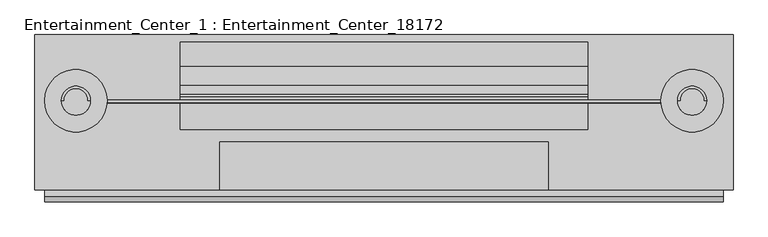
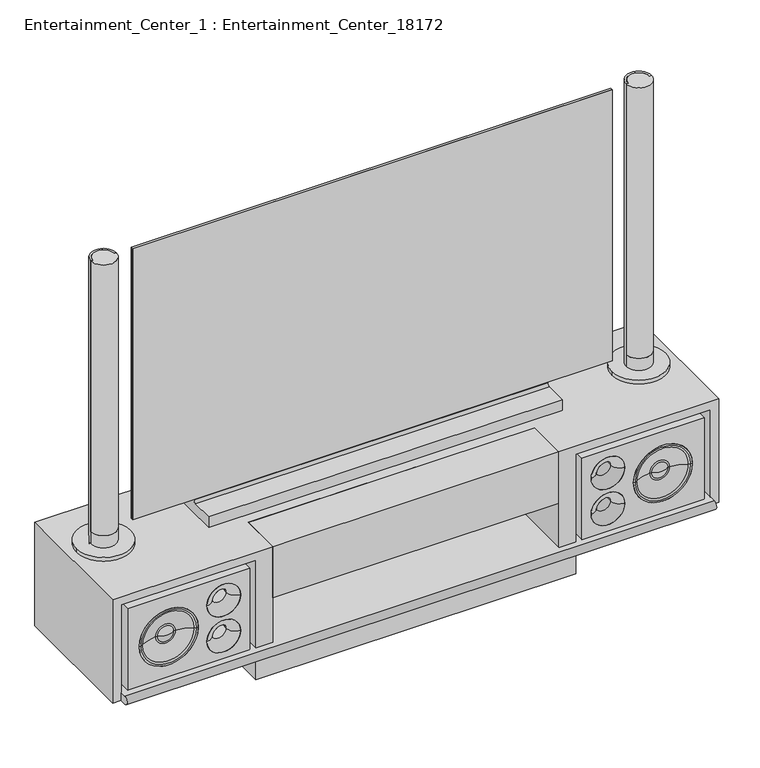
"""IFC4 building model written with IfcOpenShell, lengths in millimetres: furniture geometry, Entertainment_Center_1 : Entertainment_Center_18172."""

from ifc_helpers import new_model, si_unit, point, frame, frame_2d, origin, origin_with_axes, place, context, project, spatial, polyline, circle_curve, ellipse_curve, trimmed, segment, composite_curve, outline, extrude, faceted_brep, source, transform, mapped, element, save
from ifc_brep_helpers import plane_surface, cylinder_surface, revolved_surface, advanced_brep


def entertainment_center_1_entertainment_center_18172_277d4ec1(model_context):
    return source(origin(), model_context, "Body", "SolidModel", [
        faceted_brep([(-914.4, -406.4, 406.4), (-914.4, 0.0, 406.4), (-914.4, 0.0, 76.2), (-914.4, -406.4, 76.2), (914.4, -406.4, 406.4), (914.4, -406.4, 76.2), (914.4, 0.0, 76.2), (914.4, 0.0, 406.4), (-889.0, -406.4, 76.2), (-889.0, -406.4, 381.0), (-482.6, -406.4, 381.0), (-482.6, -406.4, 76.2), (-431.8, -406.4, 76.2), (-431.8, -406.4, 406.4), (431.8, -406.4, 406.4), (431.8, -406.4, 76.2), (482.6, -406.4, 76.2), (482.6, -406.4, 381.0), (889.0, -406.4, 381.0), (889.0, -406.4, 76.2), (889.0, -25.4, 76.2), (482.6, -25.4, 76.2), (431.8, -25.4, 76.2), (-431.8, -25.4, 76.2), (-482.6, -25.4, 76.2), (-889.0, -25.4, 76.2), (-431.8, -279.1188103, 406.4), (431.8, -279.1188103, 406.4), (-889.0, -25.4, 381.0), (-482.6, -25.4, 381.0), (889.0, -25.4, 381.0), (482.6, -25.4, 381.0), (-431.8, -25.4, 381.0), (-431.8, -279.1188103, 381.0), (431.8, -25.4, 381.0), (431.8, -279.1188103, 381.0)], [[[0, 1, 2, 3]], [[4, 5, 6, 7]], [[0, 3, 8, 9, 10, 11, 12, 13]], [[5, 4, 14, 15, 16, 17, 18, 19]], [[3, 2, 6, 5, 19, 20, 21, 16, 15, 22, 23, 12, 11, 24, 25, 8]], [[2, 1, 7, 6]], [[1, 0, 13, 26, 27, 14, 4, 7]], [[28, 9, 8, 25]], [[29, 24, 11, 10]], [[9, 28, 29, 10]], [[28, 25, 24, 29]], [[30, 20, 19, 18]], [[31, 17, 16, 21]], [[30, 18, 17, 31]], [[20, 30, 31, 21]], [[23, 32, 33, 26, 13, 12]], [[34, 22, 15, 14, 27, 35]], [[32, 34, 35, 33]], [[32, 23, 22, 34]], [[26, 33, 35, 27]]]),
        extrude(outline(composite_curve([segment(trimmed(circle_curve(frame_2d((-425.45, 88.9)), 12.7), [point((-425.45, 76.2))], [point((-425.45, 101.6))], False, "CARTESIAN"), True, "CONTINUOUS"), segment(polyline([(-425.45, 101.6), (-25.4, 101.6), (-25.4, 76.2), (-425.45, 76.2)]), True, "CONTINUOUS")], self_intersect=False)), frame((-889.0, 0.0, 0.0), z_axis=(1.0, 0.0, 0.0), x_axis=(0.0, 1.0, 0.0)), (0.0, 0.0, 1.0), 1778.0),
        extrude(outline(polyline([(-431.8, -25.4), (431.8, -25.4), (431.8, -368.0188103), (-431.8, -368.0188103), (-431.8, -25.4)])), frame((0.0, 0.0, 241.3), z_axis=(0.0, 0.0, 1.0), x_axis=(1.0, 0.0, 0.0)), (0.0, 0.0, 1.0), 10.9060017),
        extrude(outline(polyline([(-406.4, 406.4), (-279.1188103, 406.4), (-279.1188103, 400.05), (-400.05, 400.05), (-400.05, 243.0276949), (-406.4, 243.0276949), (-406.4, 406.4)])), frame((-431.8, 0.0, 0.0), z_axis=(1.0, 0.0, 0.0), x_axis=(0.0, 1.0, 0.0)), (0.0, 0.0, 1.0), 863.6),
        extrude(outline(polyline([(482.6, -25.4), (482.6, -406.4), (-482.6, -406.4), (-482.6, -25.4), (482.6, -25.4)])), origin_with_axes(), (0.0, 0.0, 1.0), 76.2),
        extrude(outline(polyline([(-723.4590197, -171.5160674), (723.4590197, -171.5160674), (723.4590197, -177.8660674), (-723.4590197, -177.8660674), (-723.4590197, -171.5160674)])), frame((0.0, 0.0, 457.2), z_axis=(0.0, 0.0, 1.0), x_axis=(1.0, 0.0, 0.0)), (0.0, 0.0, 1.0), 863.6),
        extrude(outline(composite_curve([segment(polyline([(-247.7160674, 441.1123847), (-179.0392237, 441.1123847)]), True, "CONTINUOUS"), segment(trimmed(circle_curve(frame_2d((-179.0392237, 448.6355411)), 7.5231564), [point((-179.0392237, 441.1123847))], [point((-171.5160674, 448.6355411))], True, "CARTESIAN"), True, "CONTINUOUS"), segment(polyline([(-171.5160674, 448.6355411), (-171.5160674, 658.3840106), (-161.5837628, 658.3840106), (-155.1782559, 640.7850249)]), True, "CONTINUOUS"), segment(trimmed(circle_curve(frame_2d((-495.3, 516.9908341)), 361.95), [point((-155.1782559, 640.7850249))], [point((-133.35, 516.9908341))], False, "CARTESIAN"), True, "CONTINUOUS"), segment(polyline([(-133.35, 516.9908341), (-133.35, 491.9123847)]), True, "CONTINUOUS"), segment(trimmed(circle_curve(frame_2d((-82.55, 491.9123847)), 50.8), [point((-133.35, 491.9123847))], [point((-82.55, 441.1123847))], True, "CARTESIAN"), True, "CONTINUOUS"), segment(polyline([(-82.55, 441.1123847), (-19.05, 441.1123847), (-19.05, 406.4), (-247.7160674, 406.4), (-247.7160674, 441.1123847)]), True, "CONTINUOUS")], self_intersect=False)), frame((-533.4, 0.0, 0.0), z_axis=(1.0, 0.0, 0.0), x_axis=(0.0, 1.0, 0.0)), (0.0, 0.0, 1.0), 1066.8),
        extrude(outline(polyline([(723.4590197, -179.4295839), (-723.4590197, -179.4295839), (-723.4590197, -175.7159791), (723.4590197, -175.7159791), (723.4590197, -179.4295839)])), frame((0.0, 0.0, 457.2), z_axis=(0.0, 0.0, 1.0), x_axis=(1.0, 0.0, 0.0)), (0.0, 0.0, 1.0), 863.6),
        advanced_brep(
        [(-845.3548485, -172.8664931, 406.4), (-769.1548485, -172.8664931, 406.4), (-769.1548485, -172.8664931, 1320.8), (-845.3548485, -172.8664931, 1320.8), (-839.0048485, -172.8664931, 1320.8), (-775.5048485, -172.8664931, 1320.8), (-845.3548485, -172.8664931, 457.2), (-769.1548485, -172.8664931, 457.2), (-839.0048485, -172.8664931, 457.2), (-775.5048485, -172.8664931, 457.2)],
        [
            (0, 1, circle_curve(frame((-807.2548485, -172.8664931, 406.4), z_axis=(0.0, 0.0, -1.0), x_axis=(1.0, 0.0, 0.0)), 38.1)),
            (1, 0, circle_curve(frame((-807.2548485, -172.8664931, 406.4), z_axis=(0.0, 0.0, -1.0), x_axis=(1.0, 0.0, 0.0)), 38.1)),
            (2, 3, circle_curve(frame((-807.2548485, -172.8664931, 1320.8), z_axis=(0.0, 0.0, 1.0), x_axis=(1.0, 0.0, 0.0)), 38.1)),
            (3, 4),
            (4, 5, circle_curve(frame((-807.2548485, -172.8664931, 1320.8), z_axis=(0.0, 0.0, -1.0), x_axis=(1.0, 0.0, 0.0)), 31.75)),
            (5, 2),
            (0, 6),
            (6, 3),
            (2, 7),
            (7, 1),
            (7, 6, circle_curve(frame((-807.2548485, -172.8664931, 457.2), z_axis=(0.0, 0.0, -1.0), x_axis=(1.0, 0.0, 0.0)), 38.1)),
            (8, 6),
            (7, 9),
            (9, 8, circle_curve(frame((-807.2548485, -172.8664931, 457.2), z_axis=(0.0, 0.0, 1.0), x_axis=(1.0, 0.0, 0.0)), 31.75)),
            (8, 4),
            (5, 9),
        ],
        [
            plane_surface(frame((-812.8, 0.0, 406.4), z_axis=(0.0, 0.0, -1.0), x_axis=(0.0, -1.0, 0.0))),
            plane_surface(frame((-812.8, 0.0, 1320.8), z_axis=(0.0, 0.0, 1.0), x_axis=(0.0, -1.0, 0.0))),
            cylinder_surface(frame((-807.2548485, -172.8664931, 406.4), z_axis=(0.0, 0.0, -1.0), x_axis=(1.0, 0.0, 0.0)), 38.1),
            plane_surface(frame((-807.2548485, 0.0, 457.2), z_axis=(0.0, 0.0, 1.0), x_axis=(0.0, -1.0, 0.0))),
            plane_surface(frame((-839.0048485, -172.8664931, 1320.8), z_axis=(0.0, -1.0, 0.0), x_axis=(0.0, 0.0, -1.0))),
            plane_surface(frame((-769.1548485, -172.8664931, 1320.8), z_axis=(0.0, -1.0, 0.0), x_axis=(0.0, 0.0, -1.0))),
            revolved_surface(polyline([(-775.5048485, -172.8664931, 1320.8), (-775.5048485, -172.8664931, 457.20000000000005)]), (-807.2548485, -172.8664931, 1320.8), (0.0, 0.0, 1.0)),
        ],
        [
            (0, [[1, 2]]),
            (1, [[3, 4, 5, 6]]),
            (2, [[-1, 7, 8, -3, 9, 10]]),
            (2, [[-2, -10, 11, -7]]),
            (3, [[12, -11, 13, 14]]),
            (4, [[-12, 15, -4, -8]]),
            (5, [[-13, -9, -6, 16]]),
            (6, [[-14, -16, -5, -15]]),
        ],
    ),
        extrude(outline(composite_curve([segment(trimmed(circle_curve(frame_2d((-807.2548485, -172.8664931)), 81.7451515), [point((-889.0, -172.8664931))], [point((-725.509697, -172.8664931))], False, "CARTESIAN"), True, "CONTINUOUS"), segment(trimmed(circle_curve(frame_2d((-807.2548485, -172.8664931)), 81.7451515), [point((-725.509697, -172.8664931))], [point((-889.0, -172.8664931))], False, "CARTESIAN"), True, "CONTINUOUS")], self_intersect=False)), frame((0.0, 0.0, 406.4), z_axis=(0.0, 0.0, 1.0), x_axis=(1.0, 0.0, 0.0)), (0.0, 0.0, 1.0), 12.7),
        extrude(outline(composite_curve([segment(trimmed(circle_curve(frame_2d((807.2548485, -172.8664931)), 81.7451515), [point((889.0, -172.8664931))], [point((725.509697, -172.8664931))], False, "CARTESIAN"), True, "CONTINUOUS"), segment(trimmed(circle_curve(frame_2d((807.2548485, -172.8664931)), 81.7451515), [point((725.509697, -172.8664931))], [point((889.0, -172.8664931))], False, "CARTESIAN"), True, "CONTINUOUS")], self_intersect=False)), frame((0.0, 0.0, 406.4), z_axis=(0.0, 0.0, 1.0), x_axis=(1.0, 0.0, 0.0)), (0.0, 0.0, 1.0), 12.7),
        extrude(outline(composite_curve([segment(trimmed(circle_curve(frame_2d((-807.2548485, -172.8664931)), 38.1), [point((-769.1548485, -172.8664931))], [point((-845.3548485, -172.8664931))], False, "CARTESIAN"), True, "CONTINUOUS"), segment(polyline([(-845.3548485, -172.8664931), (-839.0048485, -172.8664931)]), True, "CONTINUOUS"), segment(trimmed(circle_curve(frame_2d((-807.2548485, -172.8664931)), 31.75), [point((-839.0048485, -172.8664931))], [point((-775.5048485, -172.8664931))], False, "CARTESIAN"), True, "CONTINUOUS"), segment(polyline([(-775.5048485, -172.8664931), (-769.1548485, -172.8664931)]), True, "CONTINUOUS")], self_intersect=False)), frame((0.0, 0.0, 457.2), z_axis=(0.0, 0.0, 1.0), x_axis=(1.0, 0.0, 0.0)), (0.0, 0.0, 1.0), 863.6),
        advanced_brep(
        [(845.3548485, -172.8664931, 406.4), (769.1548485, -172.8664931, 406.4), (845.3548485, -172.8664931, 1320.8), (769.1548485, -172.8664931, 1320.8), (775.5048485, -172.8664931, 1320.8), (839.0048485, -172.8664931, 1320.8), (769.1548485, -172.8664931, 457.2), (845.3548485, -172.8664931, 457.2), (839.0048485, -172.8664931, 457.2), (775.5048485, -172.8664931, 457.2)],
        [
            (0, 1, circle_curve(frame((807.2548485, -172.8664931, 406.4), z_axis=(0.0, 0.0, -1.0), x_axis=(-1.0, 0.0, 0.0)), 38.1)),
            (1, 0, circle_curve(frame((807.2548485, -172.8664931, 406.4), z_axis=(0.0, 0.0, -1.0), x_axis=(-1.0, 0.0, 0.0)), 38.1)),
            (2, 3, circle_curve(frame((807.2548485, -172.8664931, 1320.8), z_axis=(0.0, 0.0, 1.0), x_axis=(-1.0, 0.0, 0.0)), 38.1)),
            (3, 4),
            (4, 5, circle_curve(frame((807.2548485, -172.8664931, 1320.8), z_axis=(0.0, 0.0, -1.0), x_axis=(-1.0, 0.0, 0.0)), 31.75)),
            (5, 2),
            (1, 6),
            (6, 3),
            (2, 7),
            (7, 0),
            (7, 6, circle_curve(frame((807.2548485, -172.8664931, 457.2), z_axis=(0.0, 0.0, -1.0), x_axis=(-1.0, 0.0, 0.0)), 38.1)),
            (8, 9, circle_curve(frame((807.2548485, -172.8664931, 457.2), z_axis=(0.0, 0.0, 1.0), x_axis=(-1.0, 0.0, 0.0)), 31.75)),
            (9, 6),
            (7, 8),
            (5, 8),
            (9, 4),
        ],
        [
            plane_surface(frame((812.8, 0.0, 406.4), z_axis=(0.0, 0.0, -1.0), x_axis=(0.0, 1.0, 0.0))),
            plane_surface(frame((812.8, 0.0, 1320.8), z_axis=(0.0, 0.0, 1.0), x_axis=(0.0, 1.0, 0.0))),
            cylinder_surface(frame((807.2548485, -172.8664931, 406.4), z_axis=(0.0, 0.0, -1.0), x_axis=(-1.0, 0.0, 0.0)), 38.1),
            plane_surface(frame((807.2548485, 0.0, 457.2), z_axis=(0.0, 0.0, 1.0), x_axis=(0.0, 1.0, 0.0))),
            plane_surface(frame((845.3548485, -172.8664931, 1320.8), z_axis=(0.0, -1.0, 0.0), x_axis=(0.0, 0.0, -1.0))),
            plane_surface(frame((775.5048485, -172.8664931, 1320.8), z_axis=(0.0, -1.0, 0.0), x_axis=(0.0, 0.0, -1.0))),
            revolved_surface(polyline([(775.5048485, -172.8664931, 1320.8), (775.5048485, -172.8664931, 457.20000000000005)]), (807.2548485, -172.8664931, 1320.8), (0.0, 0.0, 1.0)),
        ],
        [
            (0, [[1, 2]]),
            (1, [[3, 4, 5, 6]]),
            (2, [[-2, 7, 8, -3, 9, 10]]),
            (2, [[-1, -10, 11, -7]]),
            (3, [[12, 13, -11, 14]]),
            (4, [[-14, -9, -6, 15]]),
            (5, [[-13, 16, -4, -8]]),
            (6, [[-12, -15, -5, -16]]),
        ],
    ),
        extrude(outline(composite_curve([segment(trimmed(circle_curve(frame_2d((807.2548485, -172.8664931)), 38.1), [point((845.3548485, -172.8664931))], [point((769.1548485, -172.8664931))], False, "CARTESIAN"), True, "CONTINUOUS"), segment(polyline([(769.1548485, -172.8664931), (775.5048485, -172.8664931)]), True, "CONTINUOUS"), segment(trimmed(circle_curve(frame_2d((807.2548485, -172.8664931)), 31.75), [point((775.5048485, -172.8664931))], [point((839.0048485, -172.8664931))], False, "CARTESIAN"), True, "CONTINUOUS"), segment(polyline([(839.0048485, -172.8664931), (845.3548485, -172.8664931)]), True, "CONTINUOUS")], self_intersect=False)), frame((0.0, 0.0, 457.2), z_axis=(0.0, 0.0, 1.0), x_axis=(1.0, 0.0, 0.0)), (0.0, 0.0, 1.0), 863.6),
        extrude(outline(polyline([(-191.3302869, -321.3336205), (-191.3302869, -73.6836205), (189.6697131, -73.6836205), (189.6697131, -321.3336205), (-191.3302869, -321.3336205)])), frame((0.0, 0.0, 264.3017952), z_axis=(0.0, 0.0, 1.0), x_axis=(1.0, 0.0, 0.0)), (0.0, 0.0, 1.0), 57.15),
        extrude(outline(polyline([(-101.6, -327.3863852), (-101.6, -276.5863852), (101.6, -276.5863852), (101.6, -327.3863852), (-101.6, -327.3863852)])), frame((0.0, 0.0, 290.7540192), z_axis=(0.0, 0.0, 1.0), x_axis=(1.0, 0.0, 0.0)), (0.0, 0.0, 1.0), 19.05),
        extrude(outline(polyline([(-501.298763, -342.9), (-869.598763, -342.9), (-869.598763, -76.2), (-501.298763, -76.2), (-501.298763, -342.9)])), frame((0.0, 0.0, 101.6), z_axis=(0.0, 0.0, 1.0), x_axis=(1.0, 0.0, 0.0)), (0.0, 0.0, 1.0), 259.8201277),
        advanced_brep(
        [(-656.4895317, -406.4, 228.6), (-834.2895317, -406.4, 228.6), (-834.2895317, -342.9, 228.6), (-656.4895317, -342.9, 228.6), (-661.4072329, -406.4, 228.6), (-829.3718304, -406.4, 228.6), (-666.9861301, -403.5094482, 228.6), (-823.7929332, -403.5094482, 228.6), (-715.3754427, -388.7524859, 228.6), (-775.4036207, -388.7524859, 228.6), (-745.3895317, -398.3592917, 228.6), (-770.1255754, -389.6831477, 228.6), (-720.653488, -389.6831477, 228.6), (-745.3895317, -342.9, 228.6)],
        [
            (0, 1, circle_curve(frame((-745.3895317, -406.4, 228.6), z_axis=(0.0, 1.0, 0.0), x_axis=(-1.0, 0.0, 0.0)), 88.9)),
            (1, 2),
            (2, 3, circle_curve(frame((-745.3895317, -342.9, 228.6), z_axis=(0.0, -1.0, 0.0), x_axis=(-1.0, 0.0, 0.0)), 88.9)),
            (3, 0),
            (1, 0, circle_curve(frame((-745.3895317, -406.4, 228.6), z_axis=(0.0, 1.0, 0.0), x_axis=(-1.0, 0.0, 0.0)), 88.9)),
            (3, 2, circle_curve(frame((-745.3895317, -342.9, 228.6), z_axis=(0.0, -1.0, 0.0), x_axis=(-1.0, 0.0, 0.0)), 88.9)),
            (4, 5, circle_curve(frame((-745.3895317, -406.4, 228.6), z_axis=(0.0, 1.0, 0.0), x_axis=(-1.0, 0.0, 0.0)), 83.9822987)),
            (5, 1),
            (0, 4),
            (5, 4, circle_curve(frame((-745.3895317, -406.4, 228.6), z_axis=(0.0, 1.0, 0.0), x_axis=(-1.0, 0.0, 0.0)), 83.9822987)),
            (6, 7, circle_curve(frame((-745.3895317, -403.5094482, 228.6), z_axis=(0.0, 1.0, 0.0), x_axis=(-1.0, 0.0, 0.0)), 78.4034016)),
            (7, 5, circle_curve(frame((-827.3631505, -403.4478049, 228.6), z_axis=(0.0, 0.0, -1.0), x_axis=(1.0, 0.0, 0.0)), 3.5707494)),
            (4, 6, circle_curve(frame((-663.4159129, -403.4478049, 228.6), z_axis=(0.0, 0.0, -1.0), x_axis=(-1.0, 0.0, 0.0)), 3.5707494)),
            (7, 6, circle_curve(frame((-745.3895317, -403.5094482, 228.6), z_axis=(0.0, 1.0, 0.0), x_axis=(-1.0, 0.0, 0.0)), 78.4034016)),
            (8, 9, circle_curve(frame((-745.3895317, -388.7524859, 228.6), z_axis=(0.0, 1.0, 0.0), x_axis=(-1.0, 0.0, 0.0)), 30.014089)),
            (9, 7, circle_curve(frame((-754.4517947, -544.1700552, 228.6), z_axis=(0.0, 0.0, 1.0), x_axis=(1.0, 0.0, 0.0)), 156.8234672)),
            (6, 8, circle_curve(frame((-736.3272687, -544.1700552, 228.6), z_axis=(0.0, 0.0, 1.0), x_axis=(-1.0, 0.0, 0.0)), 156.8234672)),
            (9, 8, circle_curve(frame((-745.3895317, -388.7524859, 228.6), z_axis=(0.0, 1.0, 0.0), x_axis=(-1.0, 0.0, 0.0)), 30.014089)),
            (10, 11, circle_curve(frame((-745.3895317, -358.7594802, 228.6), z_axis=(0.0, 0.0, -1.0), x_axis=(1.0, 0.0, 0.0)), 39.5998114)),
            (11, 12, circle_curve(frame((-745.3895317, -389.6831477, 228.6), z_axis=(0.0, -1.0, 0.0), x_axis=(-1.0, 0.0, 0.0)), 24.7360437)),
            (12, 10, circle_curve(frame((-745.3895317, -358.7594802, 228.6), z_axis=(0.0, 0.0, -1.0), x_axis=(-1.0, 0.0, 0.0)), 39.5998114)),
            (12, 11, circle_curve(frame((-745.3895317, -389.6831477, 228.6), z_axis=(0.0, -1.0, 0.0), x_axis=(-1.0, 0.0, 0.0)), 24.7360437)),
            (2, 13),
            (13, 3),
            (11, 9, circle_curve(frame((-772.5432213, -387.9623269, 228.6), z_axis=(0.0, 0.0, -1.0), x_axis=(1.0, 0.0, 0.0)), 2.9675303)),
            (8, 12, circle_curve(frame((-718.2358421, -387.9623269, 228.6), z_axis=(0.0, 0.0, -1.0), x_axis=(-1.0, 0.0, 0.0)), 2.9675303)),
        ],
        [
            cylinder_surface(frame((-745.3895317, -391.7344921, 228.6), z_axis=(0.0, -1.0, 0.0), x_axis=(-1.0, 0.0, 0.0)), 88.9),
            plane_surface(frame((-745.3895317, -406.4, 228.6), z_axis=(0.0, -1.0, 0.0), x_axis=(-1.0, 0.0, 0.0))),
            revolved_surface(trimmed(ellipse_curve(frame((-827.3631505, -403.4478049, 228.6), z_axis=(0.0, 0.0, 1.0), x_axis=(1.0, 0.0, 0.0)), 3.5707494, 3.5707494), [point((-829.3718304, -406.4, 228.6))], [point((-823.7929332, -403.5094482, 228.6))], True, "CARTESIAN"), (-745.3895317, -391.7344921, 228.6), (0.0, -1.0, 0.0)),
            revolved_surface(trimmed(ellipse_curve(frame((-754.4517947, -544.1700552, 228.6), z_axis=(0.0, 0.0, -1.0), x_axis=(1.0, 0.0, 0.0)), 156.8234672, 156.8234672), [point((-823.7929332, -403.5094482, 228.6))], [point((-775.4036207, -388.7524859, 228.6))], True, "CARTESIAN"), (-745.3895317, -391.7344921, 228.6), (0.0, -1.0, 0.0)),
            revolved_surface(trimmed(ellipse_curve(frame((-745.3895317, -358.7594802, 228.6), z_axis=(0.0, 0.0, 1.0), x_axis=(1.0, 0.0, 0.0)), 39.5998114, 39.5998114), [point((-770.1255754, -389.6831477, 228.6))], [point((-745.3895317, -398.3592917, 228.6))], True, "CARTESIAN"), (-745.3895317, -391.7344921, 228.6), (0.0, -1.0, 0.0)),
            plane_surface(frame((-745.3895317, -342.9, 228.6), z_axis=(0.0, 1.0, 0.0), x_axis=(-1.0, 0.0, 0.0))),
            revolved_surface(trimmed(ellipse_curve(frame((-772.5432213, -387.9623269, 228.6), z_axis=(0.0, 0.0, 1.0), x_axis=(1.0, 0.0, 0.0)), 2.9675303, 2.9675303), [point((-775.4036207, -388.7524859, 228.6))], [point((-770.1255754, -389.6831477, 228.6))], True, "CARTESIAN"), (-745.3895317, -391.7344921, 228.6), (0.0, -1.0, 0.0)),
        ],
        [
            (0, [[1, 2, 3, 4]]),
            (0, [[5, -4, 6, -2]]),
            (1, [[7, 8, -1, 9]]),
            (1, [[10, -9, -5, -8]]),
            (2, [[11, 12, -7, 13]]),
            (2, [[14, -13, -10, -12]]),
            (3, [[15, 16, -11, 17]]),
            (3, [[18, -17, -14, -16]]),
            (4, [[19, 20, 21]]),
            (4, [[-21, 22, -19]]),
            (5, [[-3, 23, 24]]),
            (5, [[-6, -24, -23]]),
            (6, [[-20, 25, -15, 26]]),
            (6, [[-22, -26, -18, -25]]),
        ],
    ),
        extrude(outline(polyline([(361.4201277, -501.298763), (361.4201277, -869.598763), (101.6, -869.598763), (101.6, -501.298763), (361.4201277, -501.298763)]), holes=[composite_curve([segment(trimmed(circle_curve(frame_2d((228.6, -745.3895317)), 88.9), [point((228.6, -834.2895317))], [point((228.6, -656.4895317))], True, "CARTESIAN"), True, "CONTINUOUS"), segment(trimmed(circle_curve(frame_2d((228.6, -745.3895317)), 88.9), [point((228.6, -656.4895317))], [point((228.6, -834.2895317))], True, "CARTESIAN"), True, "CONTINUOUS")], self_intersect=False), composite_curve([segment(trimmed(circle_curve(frame_2d((173.1686264, -579.5939749)), 50.8), [point((173.1686264, -630.3939749))], [point((173.1686264, -528.7939749))], True, "CARTESIAN"), True, "CONTINUOUS"), segment(trimmed(circle_curve(frame_2d((173.1686264, -579.5939749)), 50.8), [point((173.1686264, -528.7939749))], [point((173.1686264, -630.3939749))], True, "CARTESIAN"), True, "CONTINUOUS")], self_intersect=False), composite_curve([segment(trimmed(circle_curve(frame_2d((287.4686264, -579.5939749)), 50.8), [point((287.4686264, -630.3939749))], [point((287.4686264, -528.7939749))], True, "CARTESIAN"), True, "CONTINUOUS"), segment(trimmed(circle_curve(frame_2d((287.4686264, -579.5939749)), 50.8), [point((287.4686264, -528.7939749))], [point((287.4686264, -630.3939749))], True, "CARTESIAN"), True, "CONTINUOUS")], self_intersect=False)]), frame((0.0, -406.4, 0.0), z_axis=(0.0, 1.0, 0.0), x_axis=(0.0, 0.0, 1.0)), (0.0, 0.0, 1.0), 63.5),
        advanced_brep(
        [(-554.8020523, -342.9, 173.1686264), (-604.3858975, -342.9, 173.1686264), (-602.8610938, -377.9369622, 173.1686264), (-556.3268561, -377.9369622, 173.1686264), (-528.7939749, -342.9, 173.1686264), (-630.3939749, -342.9, 173.1686264), (-528.7939749, -406.4, 173.1686264), (-630.3939749, -406.4, 173.1686264)],
        [
            (0, 1, circle_curve(frame((-579.5939749, -342.9, 173.1686264), z_axis=(0.0, 1.0, 0.0), x_axis=(-1.0, 0.0, 0.0)), 24.7919226)),
            (1, 2),
            (2, 3, circle_curve(frame((-579.5939749, -377.9369622, 173.1686264), z_axis=(0.0, -1.0, 0.0), x_axis=(-1.0, 0.0, 0.0)), 23.2671189)),
            (3, 0),
            (1, 0, circle_curve(frame((-579.5939749, -342.9, 173.1686264), z_axis=(0.0, 1.0, 0.0), x_axis=(-1.0, 0.0, 0.0)), 24.7919226)),
            (3, 2, circle_curve(frame((-579.5939749, -377.9369622, 173.1686264), z_axis=(0.0, -1.0, 0.0), x_axis=(-1.0, 0.0, 0.0)), 23.2671189)),
            (4, 5, circle_curve(frame((-579.5939749, -342.9, 173.1686264), z_axis=(0.0, 1.0, 0.0), x_axis=(-1.0, 0.0, 0.0)), 50.8)),
            (5, 1),
            (0, 4),
            (5, 4, circle_curve(frame((-579.5939749, -342.9, 173.1686264), z_axis=(0.0, 1.0, 0.0), x_axis=(-1.0, 0.0, 0.0)), 50.8)),
            (6, 7, circle_curve(frame((-579.5939749, -406.4, 173.1686264), z_axis=(0.0, 1.0, 0.0), x_axis=(-1.0, 0.0, 0.0)), 50.8)),
            (7, 5),
            (4, 6),
            (7, 6, circle_curve(frame((-579.5939749, -406.4, 173.1686264), z_axis=(0.0, 1.0, 0.0), x_axis=(-1.0, 0.0, 0.0)), 50.8)),
            (2, 7, circle_curve(frame((-630.1137437, -379.1229937, 173.1686264), z_axis=(0.0, 0.0, -1.0), x_axis=(1.0, 0.0, 0.0)), 27.2784457)),
            (6, 3, circle_curve(frame((-529.0742061, -379.1229937, 173.1686264), z_axis=(0.0, 0.0, -1.0), x_axis=(-1.0, 0.0, 0.0)), 27.2784457)),
        ],
        [
            revolved_surface(polyline([(-602.8610938, -377.9369622, 173.1686264), (-604.3858975, -342.9, 173.1686264)]), (-579.5939749, -374.65, 173.1686264), (0.0, -1.0, 0.0)),
            plane_surface(frame((-579.5939749, -342.9, 173.1686264), z_axis=(0.0, 1.0, 0.0), x_axis=(-1.0, 0.0, 0.0))),
            cylinder_surface(frame((-579.5939749, -374.65, 173.1686264), z_axis=(0.0, -1.0, 0.0), x_axis=(-1.0, 0.0, 0.0)), 50.8),
            revolved_surface(trimmed(ellipse_curve(frame((-630.1137437, -379.1229937, 173.1686264), z_axis=(0.0, 0.0, 1.0), x_axis=(1.0, 0.0, 0.0)), 27.2784457, 27.2784457), [point((-630.3939749, -406.4, 173.1686264))], [point((-602.8610938, -377.9369622, 173.1686264))], True, "CARTESIAN"), (-579.5939749, -374.65, 173.1686264), (0.0, -1.0, 0.0)),
        ],
        [
            (0, [[1, 2, 3, 4]]),
            (0, [[5, -4, 6, -2]]),
            (1, [[7, 8, -1, 9]]),
            (1, [[10, -9, -5, -8]]),
            (2, [[11, 12, -7, 13]]),
            (2, [[14, -13, -10, -12]]),
            (3, [[-3, 15, -11, 16]]),
            (3, [[-6, -16, -14, -15]]),
        ],
    ),
        advanced_brep(
        [(-554.8020523, -342.9, 287.4686264), (-604.3858975, -342.9, 287.4686264), (-602.8610938, -377.9369622, 287.4686264), (-556.3268561, -377.9369622, 287.4686264), (-528.7939749, -342.9, 287.4686264), (-630.3939749, -342.9, 287.4686264), (-528.7939749, -406.4, 287.4686264), (-630.3939749, -406.4, 287.4686264)],
        [
            (0, 1, circle_curve(frame((-579.5939749, -342.9, 287.4686264), z_axis=(0.0, 1.0, 0.0), x_axis=(-1.0, 0.0, 0.0)), 24.7919226)),
            (1, 2),
            (2, 3, circle_curve(frame((-579.5939749, -377.9369622, 287.4686264), z_axis=(0.0, -1.0, 0.0), x_axis=(-1.0, 0.0, 0.0)), 23.2671189)),
            (3, 0),
            (1, 0, circle_curve(frame((-579.5939749, -342.9, 287.4686264), z_axis=(0.0, 1.0, 0.0), x_axis=(-1.0, 0.0, 0.0)), 24.7919226)),
            (3, 2, circle_curve(frame((-579.5939749, -377.9369622, 287.4686264), z_axis=(0.0, -1.0, 0.0), x_axis=(-1.0, 0.0, 0.0)), 23.2671189)),
            (4, 5, circle_curve(frame((-579.5939749, -342.9, 287.4686264), z_axis=(0.0, 1.0, 0.0), x_axis=(-1.0, 0.0, 0.0)), 50.8)),
            (5, 1),
            (0, 4),
            (5, 4, circle_curve(frame((-579.5939749, -342.9, 287.4686264), z_axis=(0.0, 1.0, 0.0), x_axis=(-1.0, 0.0, 0.0)), 50.8)),
            (6, 7, circle_curve(frame((-579.5939749, -406.4, 287.4686264), z_axis=(0.0, 1.0, 0.0), x_axis=(-1.0, 0.0, 0.0)), 50.8)),
            (7, 5),
            (4, 6),
            (7, 6, circle_curve(frame((-579.5939749, -406.4, 287.4686264), z_axis=(0.0, 1.0, 0.0), x_axis=(-1.0, 0.0, 0.0)), 50.8)),
            (2, 7, circle_curve(frame((-630.1137437, -379.1229937, 287.4686264), z_axis=(0.0, 0.0, -1.0), x_axis=(1.0, 0.0, 0.0)), 27.2784457)),
            (6, 3, circle_curve(frame((-529.0742061, -379.1229937, 287.4686264), z_axis=(0.0, 0.0, -1.0), x_axis=(-1.0, 0.0, 0.0)), 27.2784457)),
        ],
        [
            revolved_surface(polyline([(-602.8610938, -377.9369622, 287.4686264), (-604.3858975, -342.9, 287.4686264)]), (-579.5939749, -374.65, 287.4686264), (0.0, -1.0, 0.0)),
            plane_surface(frame((-579.5939749, -342.9, 287.4686264), z_axis=(0.0, 1.0, 0.0), x_axis=(-1.0, 0.0, 0.0))),
            cylinder_surface(frame((-579.5939749, -374.65, 287.4686264), z_axis=(0.0, -1.0, 0.0), x_axis=(-1.0, 0.0, 0.0)), 50.8),
            revolved_surface(trimmed(ellipse_curve(frame((-630.1137437, -379.1229937, 287.4686264), z_axis=(0.0, 0.0, 1.0), x_axis=(1.0, 0.0, 0.0)), 27.2784457, 27.2784457), [point((-630.3939749, -406.4, 287.4686264))], [point((-602.8610938, -377.9369622, 287.4686264))], True, "CARTESIAN"), (-579.5939749, -374.65, 287.4686264), (0.0, -1.0, 0.0)),
        ],
        [
            (0, [[1, 2, 3, 4]]),
            (0, [[5, -4, 6, -2]]),
            (1, [[7, 8, -1, 9]]),
            (1, [[10, -9, -5, -8]]),
            (2, [[11, 12, -7, 13]]),
            (2, [[14, -13, -10, -12]]),
            (3, [[-3, 15, -11, 16]]),
            (3, [[-6, -16, -14, -15]]),
        ],
    ),
        extrude(outline(polyline([(869.598763, -342.9), (501.298763, -342.9), (501.298763, -76.2), (869.598763, -76.2), (869.598763, -342.9)])), frame((0.0, 0.0, 101.6), z_axis=(0.0, 0.0, 1.0), x_axis=(1.0, 0.0, 0.0)), (0.0, 0.0, 1.0), 259.8201277),
        advanced_brep(
        [(656.4895317, -342.9, 228.6), (834.2895317, -342.9, 228.6), (834.2895317, -406.4, 228.6), (656.4895317, -406.4, 228.6), (829.3718304, -406.4, 228.6), (661.4072329, -406.4, 228.6), (823.7929332, -403.5094482, 228.6), (666.9861301, -403.5094482, 228.6), (775.4036207, -388.7524859, 228.6), (715.3754427, -388.7524859, 228.6), (720.653488, -389.6831477, 228.6), (770.1255754, -389.6831477, 228.6), (745.3895317, -398.3592917, 228.6), (745.3895317, -342.9, 228.6)],
        [
            (0, 1, circle_curve(frame((745.3895317, -342.9, 228.6), z_axis=(0.0, -1.0, 0.0), x_axis=(1.0, 0.0, 0.0)), 88.9)),
            (1, 2),
            (2, 3, circle_curve(frame((745.3895317, -406.4, 228.6), z_axis=(0.0, 1.0, 0.0), x_axis=(1.0, 0.0, 0.0)), 88.9)),
            (3, 0),
            (1, 0, circle_curve(frame((745.3895317, -342.9, 228.6), z_axis=(0.0, -1.0, 0.0), x_axis=(1.0, 0.0, 0.0)), 88.9)),
            (3, 2, circle_curve(frame((745.3895317, -406.4, 228.6), z_axis=(0.0, 1.0, 0.0), x_axis=(1.0, 0.0, 0.0)), 88.9)),
            (2, 4),
            (4, 5, circle_curve(frame((745.3895317, -406.4, 228.6), z_axis=(0.0, 1.0, 0.0), x_axis=(1.0, 0.0, 0.0)), 83.9822987)),
            (5, 3),
            (5, 4, circle_curve(frame((745.3895317, -406.4, 228.6), z_axis=(0.0, 1.0, 0.0), x_axis=(1.0, 0.0, 0.0)), 83.9822987)),
            (4, 6, circle_curve(frame((827.3631505, -403.4478049, 228.6), z_axis=(0.0, 0.0, -1.0), x_axis=(-1.0, 0.0, 0.0)), 3.5707494)),
            (6, 7, circle_curve(frame((745.3895317, -403.5094482, 228.6), z_axis=(0.0, 1.0, 0.0), x_axis=(1.0, 0.0, 0.0)), 78.4034016)),
            (7, 5, circle_curve(frame((663.4159129, -403.4478049, 228.6), z_axis=(0.0, 0.0, -1.0), x_axis=(1.0, 0.0, 0.0)), 3.5707494)),
            (7, 6, circle_curve(frame((745.3895317, -403.5094482, 228.6), z_axis=(0.0, 1.0, 0.0), x_axis=(1.0, 0.0, 0.0)), 78.4034016)),
            (6, 8, circle_curve(frame((754.4517947, -544.1700552, 228.6), z_axis=(0.0, 0.0, 1.0), x_axis=(-1.0, 0.0, 0.0)), 156.8234672)),
            (8, 9, circle_curve(frame((745.3895317, -388.7524859, 228.6), z_axis=(0.0, 1.0, 0.0), x_axis=(1.0, 0.0, 0.0)), 30.014089)),
            (9, 7, circle_curve(frame((736.3272687, -544.1700552, 228.6), z_axis=(0.0, 0.0, 1.0), x_axis=(1.0, 0.0, 0.0)), 156.8234672)),
            (9, 8, circle_curve(frame((745.3895317, -388.7524859, 228.6), z_axis=(0.0, 1.0, 0.0), x_axis=(1.0, 0.0, 0.0)), 30.014089)),
            (10, 11, circle_curve(frame((745.3895317, -389.6831477, 228.6), z_axis=(0.0, -1.0, 0.0), x_axis=(1.0, 0.0, 0.0)), 24.7360437)),
            (11, 12, circle_curve(frame((745.3895317, -358.7594802, 228.6), z_axis=(0.0, 0.0, -1.0), x_axis=(-1.0, 0.0, 0.0)), 39.5998114)),
            (12, 10, circle_curve(frame((745.3895317, -358.7594802, 228.6), z_axis=(0.0, 0.0, -1.0), x_axis=(1.0, 0.0, 0.0)), 39.5998114)),
            (11, 10, circle_curve(frame((745.3895317, -389.6831477, 228.6), z_axis=(0.0, -1.0, 0.0), x_axis=(1.0, 0.0, 0.0)), 24.7360437)),
            (13, 1),
            (0, 13),
            (8, 11, circle_curve(frame((772.5432213, -387.9623269, 228.6), z_axis=(0.0, 0.0, -1.0), x_axis=(-1.0, 0.0, 0.0)), 2.9675303)),
            (10, 9, circle_curve(frame((718.2358421, -387.9623269, 228.6), z_axis=(0.0, 0.0, -1.0), x_axis=(1.0, 0.0, 0.0)), 2.9675303)),
        ],
        [
            cylinder_surface(frame((745.3895317, -391.7344921, 228.6), z_axis=(0.0, 1.0, 0.0), x_axis=(1.0, 0.0, 0.0)), 88.9),
            plane_surface(frame((745.3895317, -406.4, 228.6), z_axis=(0.0, -1.0, 0.0), x_axis=(1.0, 0.0, 0.0))),
            revolved_surface(trimmed(ellipse_curve(frame((827.3631505, -403.4478049, 228.6), z_axis=(0.0, 0.0, 1.0), x_axis=(-1.0, 0.0, 0.0)), 3.5707494, 3.5707494), [point((823.7929332, -403.5094482, 228.6))], [point((829.3718304, -406.4, 228.6))], True, "CARTESIAN"), (745.3895317, -391.7344921, 228.6), (0.0, 1.0, 0.0)),
            revolved_surface(trimmed(ellipse_curve(frame((754.4517947, -544.1700552, 228.6), z_axis=(0.0, 0.0, -1.0), x_axis=(-1.0, 0.0, 0.0)), 156.8234672, 156.8234672), [point((775.4036207, -388.7524859, 228.6))], [point((823.7929332, -403.5094482, 228.6))], True, "CARTESIAN"), (745.3895317, -391.7344921, 228.6), (0.0, 1.0, 0.0)),
            revolved_surface(trimmed(ellipse_curve(frame((745.3895317, -358.7594802, 228.6), z_axis=(0.0, 0.0, 1.0), x_axis=(-1.0, 0.0, 0.0)), 39.5998114, 39.5998114), [point((745.3895317, -398.3592917, 228.6))], [point((770.1255754, -389.6831477, 228.6))], True, "CARTESIAN"), (745.3895317, -391.7344921, 228.6), (0.0, 1.0, 0.0)),
            plane_surface(frame((745.3895317, -342.9, 228.6), z_axis=(0.0, 1.0, 0.0), x_axis=(1.0, 0.0, 0.0))),
            revolved_surface(trimmed(ellipse_curve(frame((772.5432213, -387.9623269, 228.6), z_axis=(0.0, 0.0, 1.0), x_axis=(-1.0, 0.0, 0.0)), 2.9675303, 2.9675303), [point((770.1255754, -389.6831477, 228.6))], [point((775.4036207, -388.7524859, 228.6))], True, "CARTESIAN"), (745.3895317, -391.7344921, 228.6), (0.0, 1.0, 0.0)),
        ],
        [
            (0, [[1, 2, 3, 4]]),
            (0, [[5, -4, 6, -2]]),
            (1, [[-3, 7, 8, 9]]),
            (1, [[-6, -9, 10, -7]]),
            (2, [[-8, 11, 12, 13]]),
            (2, [[-10, -13, 14, -11]]),
            (3, [[-12, 15, 16, 17]]),
            (3, [[-14, -17, 18, -15]]),
            (4, [[19, 20, 21]]),
            (4, [[22, -21, -20]]),
            (5, [[23, -1, 24]]),
            (5, [[-24, -5, -23]]),
            (6, [[-16, 25, -19, 26]]),
            (6, [[-18, -26, -22, -25]]),
        ],
    ),
        extrude(outline(polyline([(361.4201277, 501.298763), (101.6, 501.298763), (101.6, 869.598763), (361.4201277, 869.598763), (361.4201277, 501.298763)]), holes=[composite_curve([segment(trimmed(circle_curve(frame_2d((228.6, 745.3895317)), 88.9), [point((228.6, 834.2895317))], [point((228.6, 656.4895317))], True, "CARTESIAN"), True, "CONTINUOUS"), segment(trimmed(circle_curve(frame_2d((228.6, 745.3895317)), 88.9), [point((228.6, 656.4895317))], [point((228.6, 834.2895317))], True, "CARTESIAN"), True, "CONTINUOUS")], self_intersect=False), composite_curve([segment(trimmed(circle_curve(frame_2d((173.1686264, 579.5939749)), 50.8), [point((173.1686264, 630.3939749))], [point((173.1686264, 528.7939749))], True, "CARTESIAN"), True, "CONTINUOUS"), segment(trimmed(circle_curve(frame_2d((173.1686264, 579.5939749)), 50.8), [point((173.1686264, 528.7939749))], [point((173.1686264, 630.3939749))], True, "CARTESIAN"), True, "CONTINUOUS")], self_intersect=False), composite_curve([segment(trimmed(circle_curve(frame_2d((287.4686264, 579.5939749)), 50.8), [point((287.4686264, 630.3939749))], [point((287.4686264, 528.7939749))], True, "CARTESIAN"), True, "CONTINUOUS"), segment(trimmed(circle_curve(frame_2d((287.4686264, 579.5939749)), 50.8), [point((287.4686264, 528.7939749))], [point((287.4686264, 630.3939749))], True, "CARTESIAN"), True, "CONTINUOUS")], self_intersect=False)]), frame((0.0, -406.4, 0.0), z_axis=(0.0, 1.0, 0.0), x_axis=(0.0, 0.0, 1.0)), (0.0, 0.0, 1.0), 63.5),
        advanced_brep(
        [(556.3268561, -377.9369622, 173.1686264), (602.8610938, -377.9369622, 173.1686264), (604.3858975, -342.9, 173.1686264), (554.8020523, -342.9, 173.1686264), (630.3939749, -342.9, 173.1686264), (528.7939749, -342.9, 173.1686264), (630.3939749, -406.4, 173.1686264), (528.7939749, -406.4, 173.1686264)],
        [
            (0, 1, circle_curve(frame((579.5939749, -377.9369622, 173.1686264), z_axis=(0.0, -1.0, 0.0), x_axis=(1.0, 0.0, 0.0)), 23.2671189)),
            (1, 2),
            (2, 3, circle_curve(frame((579.5939749, -342.9, 173.1686264), z_axis=(0.0, 1.0, 0.0), x_axis=(1.0, 0.0, 0.0)), 24.7919226)),
            (3, 0),
            (1, 0, circle_curve(frame((579.5939749, -377.9369622, 173.1686264), z_axis=(0.0, -1.0, 0.0), x_axis=(1.0, 0.0, 0.0)), 23.2671189)),
            (3, 2, circle_curve(frame((579.5939749, -342.9, 173.1686264), z_axis=(0.0, 1.0, 0.0), x_axis=(1.0, 0.0, 0.0)), 24.7919226)),
            (2, 4),
            (4, 5, circle_curve(frame((579.5939749, -342.9, 173.1686264), z_axis=(0.0, 1.0, 0.0), x_axis=(1.0, 0.0, 0.0)), 50.8)),
            (5, 3),
            (5, 4, circle_curve(frame((579.5939749, -342.9, 173.1686264), z_axis=(0.0, 1.0, 0.0), x_axis=(1.0, 0.0, 0.0)), 50.8)),
            (4, 6),
            (6, 7, circle_curve(frame((579.5939749, -406.4, 173.1686264), z_axis=(0.0, 1.0, 0.0), x_axis=(1.0, 0.0, 0.0)), 50.8)),
            (7, 5),
            (7, 6, circle_curve(frame((579.5939749, -406.4, 173.1686264), z_axis=(0.0, 1.0, 0.0), x_axis=(1.0, 0.0, 0.0)), 50.8)),
            (6, 1, circle_curve(frame((630.1137437, -379.1229937, 173.1686264), z_axis=(0.0, 0.0, -1.0), x_axis=(-1.0, 0.0, 0.0)), 27.2784457)),
            (0, 7, circle_curve(frame((529.0742061, -379.1229937, 173.1686264), z_axis=(0.0, 0.0, -1.0), x_axis=(1.0, 0.0, 0.0)), 27.2784457)),
        ],
        [
            revolved_surface(polyline([(604.3858975, -342.9, 173.1686264), (602.8610938, -377.9369622, 173.1686264)]), (579.5939749, -374.65, 173.1686264), (0.0, 1.0, 0.0)),
            plane_surface(frame((579.5939749, -342.9, 173.1686264), z_axis=(0.0, 1.0, 0.0), x_axis=(1.0, 0.0, 0.0))),
            cylinder_surface(frame((579.5939749, -374.65, 173.1686264), z_axis=(0.0, 1.0, 0.0), x_axis=(1.0, 0.0, 0.0)), 50.8),
            revolved_surface(trimmed(ellipse_curve(frame((630.1137437, -379.1229937, 173.1686264), z_axis=(0.0, 0.0, 1.0), x_axis=(-1.0, 0.0, 0.0)), 27.2784457, 27.2784457), [point((602.8610938, -377.9369622, 173.1686264))], [point((630.3939749, -406.4, 173.1686264))], True, "CARTESIAN"), (579.5939749, -374.65, 173.1686264), (0.0, 1.0, 0.0)),
        ],
        [
            (0, [[1, 2, 3, 4]]),
            (0, [[5, -4, 6, -2]]),
            (1, [[-3, 7, 8, 9]]),
            (1, [[-6, -9, 10, -7]]),
            (2, [[-8, 11, 12, 13]]),
            (2, [[-10, -13, 14, -11]]),
            (3, [[-12, 15, -1, 16]]),
            (3, [[-14, -16, -5, -15]]),
        ],
    ),
        advanced_brep(
        [(556.3268561, -377.9369622, 287.4686264), (602.8610938, -377.9369622, 287.4686264), (604.3858975, -342.9, 287.4686264), (554.8020523, -342.9, 287.4686264), (630.3939749, -342.9, 287.4686264), (528.7939749, -342.9, 287.4686264), (630.3939749, -406.4, 287.4686264), (528.7939749, -406.4, 287.4686264)],
        [
            (0, 1, circle_curve(frame((579.5939749, -377.9369622, 287.4686264), z_axis=(0.0, -1.0, 0.0), x_axis=(1.0, 0.0, 0.0)), 23.2671189)),
            (1, 2),
            (2, 3, circle_curve(frame((579.5939749, -342.9, 287.4686264), z_axis=(0.0, 1.0, 0.0), x_axis=(1.0, 0.0, 0.0)), 24.7919226)),
            (3, 0),
            (1, 0, circle_curve(frame((579.5939749, -377.9369622, 287.4686264), z_axis=(0.0, -1.0, 0.0), x_axis=(1.0, 0.0, 0.0)), 23.2671189)),
            (3, 2, circle_curve(frame((579.5939749, -342.9, 287.4686264), z_axis=(0.0, 1.0, 0.0), x_axis=(1.0, 0.0, 0.0)), 24.7919226)),
            (2, 4),
            (4, 5, circle_curve(frame((579.5939749, -342.9, 287.4686264), z_axis=(0.0, 1.0, 0.0), x_axis=(1.0, 0.0, 0.0)), 50.8)),
            (5, 3),
            (5, 4, circle_curve(frame((579.5939749, -342.9, 287.4686264), z_axis=(0.0, 1.0, 0.0), x_axis=(1.0, 0.0, 0.0)), 50.8)),
            (4, 6),
            (6, 7, circle_curve(frame((579.5939749, -406.4, 287.4686264), z_axis=(0.0, 1.0, 0.0), x_axis=(1.0, 0.0, 0.0)), 50.8)),
            (7, 5),
            (7, 6, circle_curve(frame((579.5939749, -406.4, 287.4686264), z_axis=(0.0, 1.0, 0.0), x_axis=(1.0, 0.0, 0.0)), 50.8)),
            (6, 1, circle_curve(frame((630.1137437, -379.1229937, 287.4686264), z_axis=(0.0, 0.0, -1.0), x_axis=(-1.0, 0.0, 0.0)), 27.2784457)),
            (0, 7, circle_curve(frame((529.0742061, -379.1229937, 287.4686264), z_axis=(0.0, 0.0, -1.0), x_axis=(1.0, 0.0, 0.0)), 27.2784457)),
        ],
        [
            revolved_surface(polyline([(604.3858975, -342.9, 287.4686264), (602.8610938, -377.9369622, 287.4686264)]), (579.5939749, -374.65, 287.4686264), (0.0, 1.0, 0.0)),
            plane_surface(frame((579.5939749, -342.9, 287.4686264), z_axis=(0.0, 1.0, 0.0), x_axis=(1.0, 0.0, 0.0))),
            cylinder_surface(frame((579.5939749, -374.65, 287.4686264), z_axis=(0.0, 1.0, 0.0), x_axis=(1.0, 0.0, 0.0)), 50.8),
            revolved_surface(trimmed(ellipse_curve(frame((630.1137437, -379.1229937, 287.4686264), z_axis=(0.0, 0.0, 1.0), x_axis=(-1.0, 0.0, 0.0)), 27.2784457, 27.2784457), [point((602.8610938, -377.9369622, 287.4686264))], [point((630.3939749, -406.4, 287.4686264))], True, "CARTESIAN"), (579.5939749, -374.65, 287.4686264), (0.0, 1.0, 0.0)),
        ],
        [
            (0, [[1, 2, 3, 4]]),
            (0, [[5, -4, 6, -2]]),
            (1, [[-3, 7, 8, 9]]),
            (1, [[-6, -9, 10, -7]]),
            (2, [[-8, 11, 12, 13]]),
            (2, [[-10, -13, 14, -11]]),
            (3, [[-12, 15, -1, 16]]),
            (3, [[-14, -16, -5, -15]]),
        ],
    ),
    ])


if __name__ == "__main__":
    model = new_model("IFC4")
    model_context = context("Model", 3, world=origin())
    ifc_project = project(units=[si_unit("LENGTHUNIT", "METRE", prefix="MILLI")], contexts=[model_context])
    site = spatial("IfcSite", under=ifc_project)
    building = spatial("IfcBuilding", under=site)
    placement = place(None, origin())
    entertainment_center_1_entertainment_center_18172_shape = entertainment_center_1_entertainment_center_18172_277d4ec1(model_context)
    element("IfcFurniture", 1, ObjectType="Entertainment_Center_1 : Entertainment_Center_18172", at=placement, inside=building, context=model_context, shape_type="MappedRepresentation", body=[
        mapped(entertainment_center_1_entertainment_center_18172_shape, transform((0.0, 0.0, 0.0), x_axis=(1.0, 0.0, 0.0), y_axis=(0.0, 1.0, 0.0), z_axis=(0.0, 0.0, 1.0))),
    ])
    save(model, "model.ifc")

# Revit data of these elements
# Type "Entertainment_Center_1 : Entertainment_Center_18172"
#   TV Screen = tv screen
#   TV Material = Plastic, Opaque Black
#   Console Material = Plastic, Opaque White
#   Console Glass = Glass, Cast, Clear
#   Default Elevation = 0
# Element 1 (IfcFurniture, "Entertainment_Center_1 : Entertainment_Center_18172")
#   Materials on its faces: "Plastic, Opaque White", "Plastic, Opaque Black", "Linen - White", "Glass, Cast, Clear", "Speaker", "tv screen"
# Materials
#   "tv screen": colour RGB 0 0 0, transparency 0
#   "Plastic, Opaque Black": class "Plastic", colour RGB 0 0 0, transparency 0, Description = "Plastic, generic, opaque black", Cost = 0
#   "Plastic, Opaque White": class "Plastic", colour RGB 120 120 120, transparency 0, Description = "Plastic, generic, opaque white", Cost = 0
#   "Glass, Cast, Clear": class "Glass", colour RGB 236 240 239, transparency 0.85, Description = "Cast glass, clear", Cost = 0
#   "Linen - White": class "Textile", colour RGB 120 120 120, transparency 0, Description = "Linen, white", Cost = 0
#   "Speaker": class "Fabric", colour RGB 113 117 112, transparency 0
